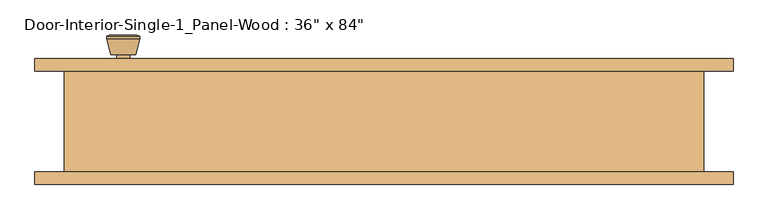
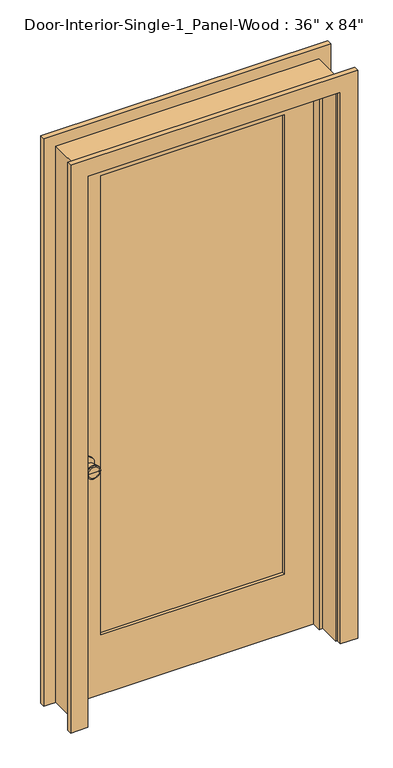
"""IFC4 building model written with IfcOpenShell, lengths in millimetres: door geometry."""

from ifc_helpers import new_model, si_unit, point, frame, frame_2d, origin, place, context, project, spatial, polyline, circle_curve, trimmed, segment, composite_curve, outline, extrude, faceted_brep, source, transform, mapped, element, save
from ifc_brep_helpers import plane_surface, cylinder_surface, revolved_surface, advanced_brep


def door_010cc4d9(model_context):
    return source(origin(), model_context, "Body", "SolidModel", [
        advanced_brep(
        [(-393.7, 32.1, 914.4), (-383.7, 32.1, 914.4), (-403.7, 32.1, 914.4), (-373.2241324, -16.9, 914.4), (-393.7, -16.9, 914.4), (-414.1758676, -16.9, 914.4), (-368.7, -15.0721319, 914.4), (-418.7, -15.0721319, 914.4), (-368.7, -11.6084537, 914.4), (-418.7, -11.6084537, 914.4), (-375.063764, 13.1, 914.4), (-412.336236, 13.1, 914.4), (-383.7, 13.1, 914.4), (-403.7, 13.1, 914.4)],
        [
            (0, 1),
            (1, 2, circle_curve(frame((-393.7, 32.1, 914.4), z_axis=(0.0, 1.0, 0.0), x_axis=(-1.0, 0.0, 0.0)), 10.0)),
            (2, 0),
            (2, 1, circle_curve(frame((-393.7, 32.1, 914.4), z_axis=(0.0, 1.0, 0.0), x_axis=(-1.0, 0.0, 0.0)), 10.0)),
            (3, 4),
            (4, 5),
            (5, 3, circle_curve(frame((-393.7, -16.9, 914.4), z_axis=(0.0, -1.0, 0.0), x_axis=(-1.0, 0.0, 0.0)), 20.4758676)),
            (3, 5, circle_curve(frame((-393.7, -16.9, 914.4), z_axis=(0.0, -1.0, 0.0), x_axis=(-1.0, 0.0, 0.0)), 20.4758676)),
            (6, 3),
            (5, 7),
            (7, 6, circle_curve(frame((-393.7, -15.0721319, 914.4), z_axis=(0.0, -1.0, 0.0), x_axis=(-1.0, 0.0, 0.0)), 25.0)),
            (6, 7, circle_curve(frame((-393.7, -15.0721319, 914.4), z_axis=(0.0, -1.0, 0.0), x_axis=(-1.0, 0.0, 0.0)), 25.0)),
            (8, 6),
            (7, 9),
            (9, 8, circle_curve(frame((-393.7, -11.6084537, 914.4), z_axis=(0.0, -1.0, 0.0), x_axis=(-1.0, 0.0, 0.0)), 25.0)),
            (8, 9, circle_curve(frame((-393.7, -11.6084537, 914.4), z_axis=(0.0, -1.0, 0.0), x_axis=(-1.0, 0.0, 0.0)), 25.0)),
            (10, 8),
            (9, 11),
            (11, 10, circle_curve(frame((-393.7, 13.1, 914.4), z_axis=(0.0, -1.0, 0.0), x_axis=(-1.0, 0.0, 0.0)), 18.636236)),
            (10, 11, circle_curve(frame((-393.7, 13.1, 914.4), z_axis=(0.0, -1.0, 0.0), x_axis=(-1.0, 0.0, 0.0)), 18.636236)),
            (12, 10),
            (11, 13),
            (13, 12, circle_curve(frame((-393.7, 13.1, 914.4), z_axis=(0.0, -1.0, 0.0), x_axis=(-1.0, 0.0, 0.0)), 10.0)),
            (12, 13, circle_curve(frame((-393.7, 13.1, 914.4), z_axis=(0.0, -1.0, 0.0), x_axis=(-1.0, 0.0, 0.0)), 10.0)),
            (1, 12),
            (13, 2),
        ],
        [
            plane_surface(frame((-393.7, 32.1, 914.4), z_axis=(0.0, 1.0, 0.0), x_axis=(-1.0, 0.0, 0.0))),
            plane_surface(frame((-393.7, -16.9, 914.4), z_axis=(0.0, -1.0, 0.0), x_axis=(-1.0, 0.0, 0.0))),
            revolved_surface(polyline([(-414.1758676, -16.9, 914.4), (-418.7, -15.0721319, 914.4)]), (-393.7, 32.1, 914.4), (0.0, 1.0, 0.0)),
            cylinder_surface(frame((-393.7, 32.1, 914.4), z_axis=(0.0, 1.0, 0.0), x_axis=(-1.0, 0.0, 0.0)), 25.0),
            revolved_surface(polyline([(-418.7, -11.6084537, 914.4), (-412.336236, 13.1, 914.4)]), (-393.7, 32.1, 914.4), (0.0, 1.0, 0.0)),
            plane_surface(frame((-393.7, 13.1, 914.4), z_axis=(0.0, 1.0, 0.0), x_axis=(-1.0, 0.0, 0.0))),
            cylinder_surface(frame((-393.7, 32.1, 914.4), z_axis=(0.0, 1.0, 0.0), x_axis=(-1.0, 0.0, 0.0)), 10.0),
        ],
        [
            (0, [[1, 2, 3]]),
            (0, [[-3, 4, -1]]),
            (1, [[5, 6, 7]]),
            (1, [[-6, -5, 8]]),
            (2, [[9, -7, 10, 11]]),
            (2, [[-10, -8, -9, 12]]),
            (3, [[13, -11, 14, 15]]),
            (3, [[-14, -12, -13, 16]]),
            (4, [[17, -15, 18, 19]]),
            (4, [[-18, -16, -17, 20]]),
            (5, [[21, -19, 22, 23]]),
            (5, [[-22, -20, -21, 24]]),
            (6, [[25, -23, 26, -2]]),
            (6, [[-26, -24, -25, -4]]),
        ],
    ),
        extrude(outline(composite_curve([segment(trimmed(circle_curve(frame_2d((914.4, -393.7)), 30.0), [point((914.4, -423.7))], [point((914.4, -363.7))], False, "CARTESIAN"), True, "CONTINUOUS"), segment(trimmed(circle_curve(frame_2d((914.4, -393.7)), 30.0), [point((914.4, -363.7))], [point((914.4, -423.7))], False, "CARTESIAN"), True, "CONTINUOUS")], self_intersect=False)), frame((0.0, 32.1, 0.0), z_axis=(0.0, 1.0, 0.0), x_axis=(0.0, 0.0, 1.0)), (0.0, 0.0, 1.0), 6.0),
        advanced_brep(
        [(-393.7, 79.025, 914.4), (-403.7, 79.025, 914.4), (-383.7, 79.025, 914.4), (-373.2241324, 128.025, 914.4), (-414.1758676, 128.025, 914.4), (-393.7, 128.025, 914.4), (-368.7, 126.1971319, 914.4), (-418.7, 126.1971319, 914.4), (-368.7, 122.7334537, 914.4), (-418.7, 122.7334537, 914.4), (-375.063764, 98.025, 914.4), (-412.336236, 98.025, 914.4), (-383.7, 98.025, 914.4), (-403.7, 98.025, 914.4)],
        [
            (0, 1),
            (1, 2, circle_curve(frame((-393.7, 79.025, 914.4), z_axis=(0.0, -1.0, 0.0), x_axis=(-1.0, 0.0, 0.0)), 10.0)),
            (2, 0),
            (2, 1, circle_curve(frame((-393.7, 79.025, 914.4), z_axis=(0.0, -1.0, 0.0), x_axis=(-1.0, 0.0, 0.0)), 10.0)),
            (3, 4, circle_curve(frame((-393.7, 128.025, 914.4), z_axis=(0.0, 1.0, 0.0), x_axis=(-1.0, 0.0, 0.0)), 20.4758676)),
            (4, 5),
            (5, 3),
            (4, 3, circle_curve(frame((-393.7, 128.025, 914.4), z_axis=(0.0, 1.0, 0.0), x_axis=(-1.0, 0.0, 0.0)), 20.4758676)),
            (6, 7, circle_curve(frame((-393.7, 126.1971319, 914.4), z_axis=(0.0, 1.0, 0.0), x_axis=(-1.0, 0.0, 0.0)), 25.0)),
            (7, 4),
            (3, 6),
            (7, 6, circle_curve(frame((-393.7, 126.1971319, 914.4), z_axis=(0.0, 1.0, 0.0), x_axis=(-1.0, 0.0, 0.0)), 25.0)),
            (8, 9, circle_curve(frame((-393.7, 122.7334537, 914.4), z_axis=(0.0, 1.0, 0.0), x_axis=(-1.0, 0.0, 0.0)), 25.0)),
            (9, 7),
            (6, 8),
            (9, 8, circle_curve(frame((-393.7, 122.7334537, 914.4), z_axis=(0.0, 1.0, 0.0), x_axis=(-1.0, 0.0, 0.0)), 25.0)),
            (10, 11, circle_curve(frame((-393.7, 98.025, 914.4), z_axis=(0.0, 1.0, 0.0), x_axis=(-1.0, 0.0, 0.0)), 18.636236)),
            (11, 9),
            (8, 10),
            (11, 10, circle_curve(frame((-393.7, 98.025, 914.4), z_axis=(0.0, 1.0, 0.0), x_axis=(-1.0, 0.0, 0.0)), 18.636236)),
            (12, 13, circle_curve(frame((-393.7, 98.025, 914.4), z_axis=(0.0, 1.0, 0.0), x_axis=(-1.0, 0.0, 0.0)), 10.0)),
            (13, 11),
            (10, 12),
            (13, 12, circle_curve(frame((-393.7, 98.025, 914.4), z_axis=(0.0, 1.0, 0.0), x_axis=(-1.0, 0.0, 0.0)), 10.0)),
            (1, 13),
            (12, 2),
        ],
        [
            plane_surface(frame((-393.7, 79.025, 914.4), z_axis=(0.0, -1.0, 0.0), x_axis=(-1.0, 0.0, 0.0))),
            plane_surface(frame((-393.7, 128.025, 914.4), z_axis=(0.0, 1.0, 0.0), x_axis=(-1.0, 0.0, 0.0))),
            revolved_surface(polyline([(-414.1758676, 128.025, 914.4), (-418.7, 126.1971319, 914.4)]), (-393.7, 79.025, 914.4), (0.0, -1.0, 0.0)),
            cylinder_surface(frame((-393.7, 79.025, 914.4), z_axis=(0.0, -1.0, 0.0), x_axis=(-1.0, 0.0, 0.0)), 25.0),
            revolved_surface(polyline([(-418.7, 122.7334537, 914.4), (-412.336236, 98.025, 914.4)]), (-393.7, 79.025, 914.4), (0.0, -1.0, 0.0)),
            plane_surface(frame((-393.7, 98.025, 914.4), z_axis=(0.0, -1.0, 0.0), x_axis=(-1.0, 0.0, 0.0))),
            cylinder_surface(frame((-393.7, 79.025, 914.4), z_axis=(0.0, -1.0, 0.0), x_axis=(-1.0, 0.0, 0.0)), 10.0),
        ],
        [
            (0, [[1, 2, 3]]),
            (0, [[-3, 4, -1]]),
            (1, [[5, 6, 7]]),
            (1, [[8, -7, -6]]),
            (2, [[9, 10, -5, 11]]),
            (2, [[12, -11, -8, -10]]),
            (3, [[13, 14, -9, 15]]),
            (3, [[16, -15, -12, -14]]),
            (4, [[17, 18, -13, 19]]),
            (4, [[20, -19, -16, -18]]),
            (5, [[21, 22, -17, 23]]),
            (5, [[24, -23, -20, -22]]),
            (6, [[-2, 25, -21, 26]]),
            (6, [[-4, -26, -24, -25]]),
        ],
    ),
        extrude(outline(composite_curve([segment(trimmed(circle_curve(frame_2d((914.4, -393.7)), 30.0), [point((914.4, -423.7))], [point((914.4, -363.7))], False, "CARTESIAN"), True, "CONTINUOUS"), segment(trimmed(circle_curve(frame_2d((914.4, -393.7)), 30.0), [point((914.4, -363.7))], [point((914.4, -423.7))], False, "CARTESIAN"), True, "CONTINUOUS")], self_intersect=False)), frame((0.0, 73.025, 0.0), z_axis=(0.0, 1.0, 0.0), x_axis=(0.0, 0.0, 1.0)), (0.0, 0.0, 1.0), 6.0),
        faceted_brep([(482.6, 73.025, 0.0), (482.6, -79.375, 0.0), (457.2, -79.375, 0.0), (457.2, 3.175, 0.0), (444.5, 3.175, 0.0), (444.5, 38.1, 0.0), (457.2, 38.1, 0.0), (457.2, 73.025, 0.0), (482.6, 73.025, 2159.0), (482.6, -79.375, 2159.0), (-482.6, -79.375, 2159.0), (-482.6, -79.375, 0.0), (-457.2, -79.375, 0.0), (-457.2, -79.375, 2133.6), (457.2, -79.375, 2133.6), (457.2, 3.175, 2133.6), (-457.2, 3.175, 2133.6), (-457.2, 3.175, 0.0), (-444.5, 3.175, 0.0), (-444.5, 3.175, 2120.9), (444.5, 3.175, 2120.9), (444.5, 38.1, 2120.9), (-444.5, 38.1, 2120.9), (-444.5, 38.1, 0.0), (-457.2, 38.1, 0.0), (-457.2, 38.1, 2133.6), (457.2, 38.1, 2133.6), (457.2, 73.025, 2133.6), (-457.2, 73.025, 2133.6), (-457.2, 73.025, 0.0), (-482.6, 73.025, 0.0), (-482.6, 73.025, 2159.0)], [[[0, 1, 2, 3, 4, 5, 6, 7]], [[1, 0, 8, 9]], [[2, 1, 9, 10, 11, 12, 13, 14]], [[3, 2, 14, 15]], [[4, 3, 15, 16, 17, 18, 19, 20]], [[5, 4, 20, 21]], [[6, 5, 21, 22, 23, 24, 25, 26]], [[7, 6, 26, 27]], [[0, 7, 27, 28, 29, 30, 31, 8]], [[9, 8, 31, 10]], [[15, 14, 13, 16]], [[21, 20, 19, 22]], [[27, 26, 25, 28]], [[30, 29, 24, 23, 18, 17, 12, 11]], [[10, 31, 30, 11]], [[16, 13, 12, 17]], [[22, 19, 18, 23]], [[28, 25, 24, 29]]]),
        extrude(outline(polyline([(2133.6, -457.2), (0.0, -457.2), (0.0, 457.2), (2133.6, 457.2), (2133.6, -457.2)]), holes=[polyline([(2014.5375, -336.55), (2014.5375, 336.55), (231.775, 336.55), (231.775, -336.55), (2014.5375, -336.55)])]), frame((0.0, 38.1, 0.0), z_axis=(0.0, 1.0, 0.0), x_axis=(0.0, 0.0, 1.0)), (0.0, 0.0, 1.0), 34.925),
        extrude(outline(polyline([(336.55, 49.7416667), (-336.55, 49.7416667), (-336.55, 61.3833333), (336.55, 61.3833333), (336.55, 49.7416667)])), frame((0.0, 0.0, 231.775), z_axis=(0.0, 0.0, 1.0), x_axis=(1.0, 0.0, 0.0)), (0.0, 0.0, 1.0), 1782.7625),
        extrude(outline(polyline([(0.0, 463.55), (0.0, 527.05), (2203.45, 527.05), (2203.45, -527.05), (0.0, -527.05), (0.0, -463.55), (2139.95, -463.55), (2139.95, 463.55), (0.0, 463.55)])), frame((0.0, 73.025, 0.0), z_axis=(0.0, 1.0, 0.0), x_axis=(0.0, 0.0, 1.0)), (0.0, 0.0, 1.0), 19.05),
        extrude(outline(polyline([(0.0, 463.55), (0.0, 527.05), (2203.45, 527.05), (2203.45, -527.05), (0.0, -527.05), (0.0, -463.55), (2139.95, -463.55), (2139.95, 463.55), (0.0, 463.55)])), frame((0.0, -98.425, 0.0), z_axis=(0.0, 1.0, 0.0), x_axis=(0.0, 0.0, 1.0)), (0.0, 0.0, 1.0), 19.05),
    ])


if __name__ == "__main__":
    model = new_model("IFC4")
    model_context = context("Model", 3, world=origin())
    ifc_project = project(units=[si_unit("LENGTHUNIT", "METRE", prefix="MILLI")], contexts=[model_context])
    site = spatial("IfcSite", under=ifc_project)
    building = spatial("IfcBuilding", under=site)
    placement = place(None, origin())
    door_shape = door_010cc4d9(model_context)
    element("IfcDoor", 1, ObjectType="Door-Interior-Single-1_Panel-Wood : 36\" x 84\"", at=placement, inside=building, context=model_context, shape_type="MappedRepresentation", body=[
        mapped(door_shape, transform((0.0, 0.0, 0.0), x_axis=(1.0, 0.0, 0.0), y_axis=(0.0, 1.0, 0.0), z_axis=(0.0, 0.0, 1.0))),
    ])
    save(model, "model.ifc")

# Revit data of these elements
# Type "Door-Interior-Single-1_Panel-Wood : 36\" x 84\""
#   Type Mark = "8"
#   Assembly Code = "C1020300"
#   Analytic Construction = "Wooden"
#   Top Rail = 0' - 4 11/16"
#   Thickness = 0' - 1 3/8"
#   Thermal Resistance (R) = 2.5876 (h·ft²·°F)/BTU
#   Swing Angle [instance default] = 90.00°
#   Stiles = 0' - 4 3/4"
#   Rough Width = 3' - 2"
#   Rough Height = 7' - 1"
#   Height = 7' - 0"
#   Width = 3' - 0"
#   Heat Transfer Coefficient (U) = 0.3865 BTU/(h·ft²·°F)
#   Bottom Rail = 0' - 9 1/8"
#   Trim Material = Cherry
#   Panel Material = Cherry
#   Frame Material = Cherry
#   Door Handle Material = Aluminum
#   Visual Light Transmittance = 0
#   Solar Heat Gain Coefficient = 0
#   Wall Closure = (empty or 0)
#   Function = (empty or 0)
# Element 1 (IfcDoor, "Door-Interior-Single-1_Panel-Wood : 36\" x 84\"")
#   Materials on its faces: "Cherry", "Aluminum"
# Materials
#   "Cherry": class "Wood", colour RGB 226 177 128, transparency 0, Description = "Prunus Serotina", Cost = 0
#   "Aluminum": class "Metal", colour RGB 247 247 247, transparency 0, Description = "Aluminum 6061", Cost = 0
